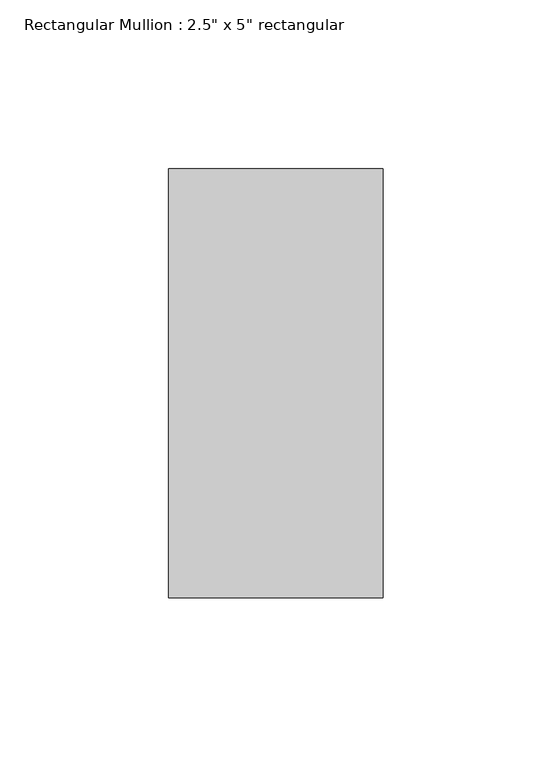
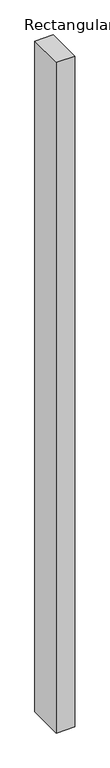
"""IFC4 building model written with IfcOpenShell, lengths in millimetres: member geometry."""

from ifc_helpers import new_model, si_unit, frame, origin, place, context, project, spatial, polyline, outline, extrude, source, transform, mapped, element, save


def member_f0fea5a5(model_context):
    return source(origin(), model_context, "Body", "SweptSolid", [
        extrude(outline(polyline([(31.75, 63.5), (31.75, -63.5), (-31.75, -63.5), (-31.75, 63.5), (31.75, 63.5)])), frame((0.0, 0.0, -2438.4), z_axis=(0.0, 0.0, 1.0), x_axis=(1.0, 0.0, 0.0)), (0.0, 0.0, 1.0), 2438.4),
    ])


if __name__ == "__main__":
    model = new_model("IFC4")
    model_context = context("Model", 3, world=origin())
    ifc_project = project(units=[si_unit("LENGTHUNIT", "METRE", prefix="MILLI")], contexts=[model_context])
    site = spatial("IfcSite", under=ifc_project)
    building = spatial("IfcBuilding", under=site)
    placement = place(None, origin())
    member_shape = member_f0fea5a5(model_context)
    element("IfcMember", 1, ObjectType="Rectangular Mullion : 2.5\" x 5\" rectangular", at=placement, inside=building, context=model_context, shape_type="MappedRepresentation", body=[
        mapped(member_shape, transform((0.0, 0.0, 0.0), x_axis=(1.0, 0.0, 0.0), y_axis=(0.0, 1.0, 0.0), z_axis=(0.0, 0.0, 1.0))),
    ])
    save(model, "model.ifc")

# Revit data of these elements
# Type "Rectangular Mullion : 2.5\" x 5\" rectangular"
#   built-in parameter 1007304 = 0.416667 (stored number, unit not read)
#   built-in parameter 1007301 = 0.104167 (stored number, unit not read)
#   built-in parameter 1007300 = 0.104167 (stored number, unit not read)
# Element 1 (IfcMember, "Rectangular Mullion : 2.5\" x 5\" rectangular")
#   Materials on its faces: "Iron, Ductile"
# Materials
#   "Iron, Ductile": class "Metal", colour RGB 0 0 0, transparency 0, Description = "Ductile cast iron", Cost = 0
